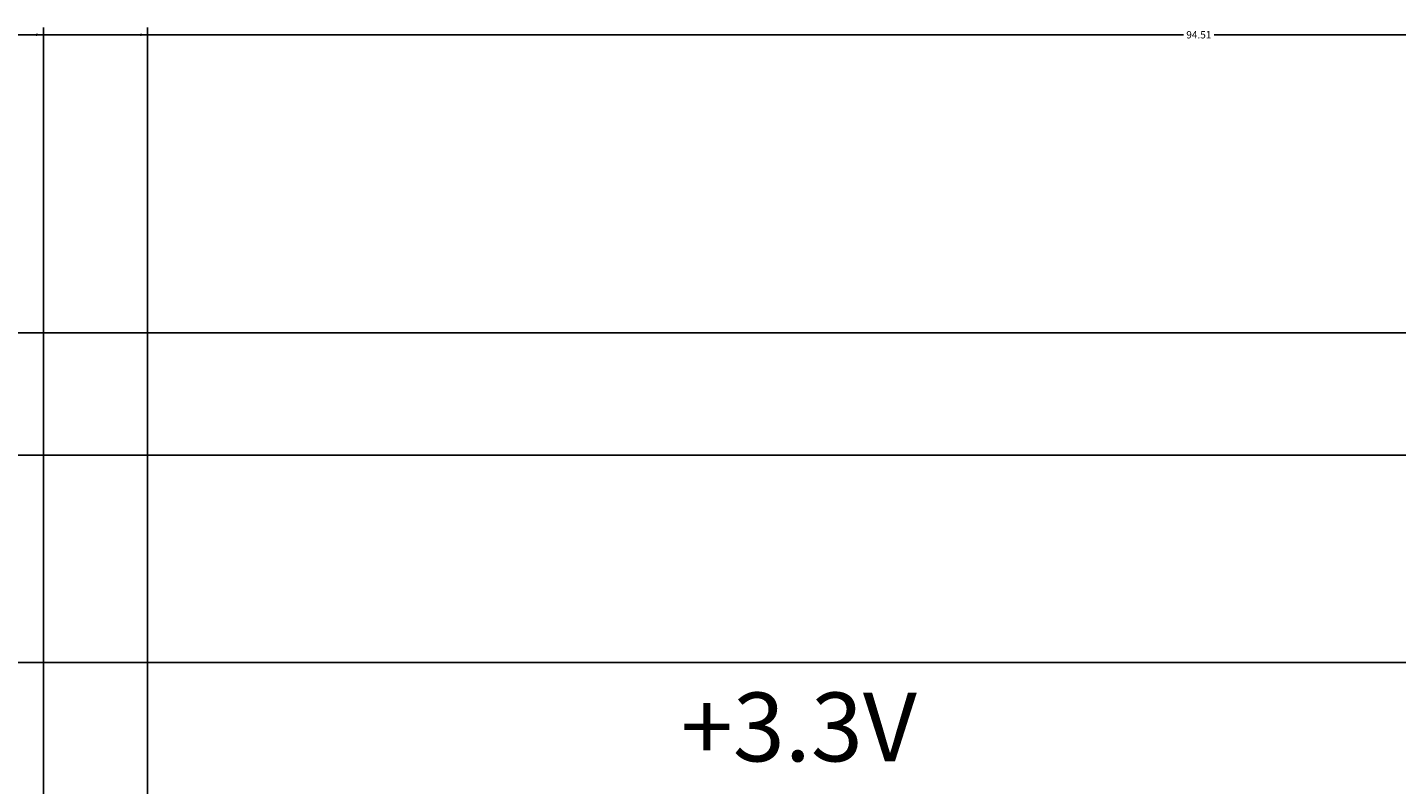
# Model space of a CAD drawing. Units: inches. Extents: x 23 to 132, y 5 to 105.
# Tile 6 of 14: x 47 to 81, y 87 to 105. Entities that reach past the tile are written whole.
import ezdxf

# ---------------------------------------------------------------- set-up
doc = ezdxf.new("R2010")
doc.units = ezdxf.units.IN
doc.header["$MEASUREMENT"] = 0
doc.layers.add('A-ANNO-DIMS', color=2, linetype='Continuous', lineweight=18)
doc.layers.add('E-ANNO-IDEN', color=4, linetype='Continuous', lineweight=18)
doc.styles.get("Standard").update_dxf_attribs({"font": 'arial.ttf'})
doc.dimstyles.get("Standard").update_dxf_attribs({"dimtxt": 0.18, "dimasz": 0.18, "dimexe": 0.18, "dimexo": 0.0625, "dimgap": 0.09, "dimtad": 0, "dimtih": 1, "dimtoh": 1, "dimdec": 4, "dimzin": 0, "dimdsep": 46, "dimtxsty": 'Standard', "dimcen": 0.09, "dimadec": 0, "dimazin": 0, "dimtfac": 1, "dimtdec": 4, "dimtofl": 0, "dimtmove": 0, "dimatfit": 3, "dimfxl": 1, "dimtolj": 1, "dimtzin": 0, "dimarcsym": 0})

# ---------------------------------------------------------------- blocks, each defined once
blk = doc.blocks.new('*D2')
at = {"layer": 'A-ANNO-DIMS', "color": 0, "lineweight": -2, "transparency": 16777216}
for p, q in [((28.697, 66.272), (28.697, 105.232)), ((123.211, 99.539), (123.211, 105.232)), ((28.877, 105.052), (75.577, 105.052)), ((123.031, 105.052), (76.33, 105.052))]:
    blk.add_line(p, q, dxfattribs=at)
at = {"layer": 'A-ANNO-DIMS', "color": 0, "transparency": 16777216}
for points in [[(28.877, 105.082), (28.877, 105.022), (28.697, 105.052)], [(123.031, 105.082), (123.031, 105.022), (123.211, 105.052)]]:
    blk.add_solid(points, dxfattribs=at)
at = {"layer": 'Defpoints', "color": 0, "transparency": 16777216}
for p in [(123.211, 105.052), (123.211, 99.477), (28.697, 66.21)]:
    blk.add_point(p, dxfattribs=at)
at = {"layer": 'A-ANNO-DIMS', "color": 0, "transparency": 16777216, "insert": (75.954, 105.052), "char_height": 0.18, "attachment_point": 5}
blk.add_mtext('\\A1;94.51', dxfattribs=at)
blk = doc.blocks.new('*D3')
at = {"layer": 'A-ANNO-DIMS', "color": 0, "lineweight": -2, "transparency": 16777216}
for p, q in [((121.409, 99.285), (129.239, 99.285)), ((129.059, 99.105), (129.059, 55.423)), ((129.059, 11.378), (129.059, 55.06)), ((72.981, 11.198), (129.239, 11.198))]:
    blk.add_line(p, q, dxfattribs=at)
at = {"layer": 'A-ANNO-DIMS', "color": 0, "transparency": 16777216}
for points in [[(129.029, 99.105), (129.089, 99.105), (129.059, 99.285)], [(129.029, 11.378), (129.089, 11.378), (129.059, 11.198)]]:
    blk.add_solid(points, dxfattribs=at)
at = {"layer": 'Defpoints', "color": 0, "transparency": 16777216}
for p in [(121.346, 99.285), (129.059, 99.285), (72.919, 11.198)]:
    blk.add_point(p, dxfattribs=at)
at = {"layer": 'A-ANNO-DIMS', "color": 0, "transparency": 16777216, "insert": (129.059, 55.241), "char_height": 0.18, "attachment_point": 5}
blk.add_mtext('\\A1;88.09', dxfattribs=at)
blk = doc.blocks.new('*D7')
at = {"layer": 'A-ANNO-DIMS', "color": 0, "lineweight": -2, "transparency": 16777216}
for p, q in [((30.295, 73.877), (30.295, 105.232)), ((50.265, 77.157), (50.265, 105.232)), ((30.475, 105.052), (39.895, 105.052)), ((50.085, 105.052), (40.665, 105.052))]:
    blk.add_line(p, q, dxfattribs=at)
at = {"layer": 'A-ANNO-DIMS', "color": 0, "transparency": 16777216}
for points in [[(30.475, 105.082), (30.475, 105.022), (30.295, 105.052)], [(50.085, 105.082), (50.085, 105.022), (50.265, 105.052)]]:
    blk.add_solid(points, dxfattribs=at)
at = {"layer": 'Defpoints', "color": 0, "transparency": 16777216}
for p in [(50.265, 105.052), (50.265, 77.095), (30.295, 73.814)]:
    blk.add_point(p, dxfattribs=at)
at = {"layer": 'A-ANNO-DIMS', "color": 0, "transparency": 16777216, "insert": (40.28, 105.052), "char_height": 0.18, "attachment_point": 5}
blk.add_mtext('\\A1;19.97', dxfattribs=at)
blk = doc.blocks.new('*D48')
at = {"layer": 'A-ANNO-DIMS', "color": 0, "lineweight": -2, "transparency": 16777216}
for p, q in [((41.783, 75.637), (41.783, 105.232)), ((47.72, 75.683), (47.72, 105.232)), ((41.963, 105.052), (44.358, 105.052)), ((47.54, 105.052), (45.145, 105.052))]:
    blk.add_line(p, q, dxfattribs=at)
at = {"layer": 'A-ANNO-DIMS', "color": 0, "transparency": 16777216}
for points in [[(41.963, 105.082), (41.963, 105.022), (41.783, 105.052)], [(47.54, 105.082), (47.54, 105.022), (47.72, 105.052)]]:
    blk.add_solid(points, dxfattribs=at)
at = {"layer": 'Defpoints', "color": 0, "transparency": 16777216}
for p in [(47.72, 105.052), (41.783, 75.575), (47.72, 75.621)]:
    blk.add_point(p, dxfattribs=at)
at = {"layer": 'A-ANNO-DIMS', "color": 0, "transparency": 16777216, "insert": (44.752, 105.052), "char_height": 0.18, "attachment_point": 5}
blk.add_mtext('\\A1;5.937', dxfattribs=at)
blk = doc.blocks.new('*D85')
at = {"layer": 'A-ANNO-DIMS', "color": 0, "lineweight": -2, "transparency": 16777216}
for p, q in [((106.903, 97.776), (22.942, 97.776)), ((23.122, 97.596), (23.122, 87.606)), ((23.122, 77.251), (23.122, 87.242)), ((106.964, 77.071), (22.942, 77.071))]:
    blk.add_line(p, q, dxfattribs=at)
at = {"layer": 'A-ANNO-DIMS', "color": 0, "transparency": 16777216}
for points in [[(23.092, 97.596), (23.152, 97.596), (23.122, 97.776)], [(23.092, 77.251), (23.152, 77.251), (23.122, 77.071)]]:
    blk.add_solid(points, dxfattribs=at)
at = {"layer": 'Defpoints', "color": 0, "transparency": 16777216}
for p in [(23.122, 97.776), (106.965, 97.776), (107.026, 77.071)]:
    blk.add_point(p, dxfattribs=at)
at = {"layer": 'A-ANNO-DIMS', "color": 0, "transparency": 16777216, "insert": (23.122, 87.424), "char_height": 0.18, "attachment_point": 5}
blk.add_mtext('\\A1;20.705', dxfattribs=at)
blk = doc.blocks.new('*D88')
at = {"layer": 'A-ANNO-DIMS', "color": 0, "lineweight": -2, "transparency": 16777216}
for p, q in [((110.027, 89.722), (22.942, 89.722)), ((23.122, 89.542), (23.122, 87.554)), ((23.122, 85.201), (23.122, 87.19)), ((110.027, 85.021), (22.942, 85.021))]:
    blk.add_line(p, q, dxfattribs=at)
at = {"layer": 'A-ANNO-DIMS', "color": 0, "transparency": 16777216}
for points in [[(23.092, 89.542), (23.152, 89.542), (23.122, 89.722)], [(23.092, 85.201), (23.152, 85.201), (23.122, 85.021)]]:
    blk.add_solid(points, dxfattribs=at)
at = {"layer": 'Defpoints', "color": 0, "transparency": 16777216}
for p in [(23.122, 89.722), (110.089, 89.722), (110.089, 85.021)]:
    blk.add_point(p, dxfattribs=at)
at = {"layer": 'A-ANNO-DIMS', "color": 0, "transparency": 16777216, "insert": (23.122, 87.372), "char_height": 0.18, "attachment_point": 5}
blk.add_mtext('\\A1;4.702', dxfattribs=at)
blk = doc.blocks.new('*D89')
at = {"layer": 'A-ANNO-DIMS', "color": 0, "lineweight": -2, "transparency": 16777216}
for p, q in [((110.298, 94.783), (22.942, 94.783)), ((23.122, 94.603), (23.122, 92.435)), ((23.122, 89.902), (23.122, 92.071)), ((110.027, 89.722), (22.942, 89.722))]:
    blk.add_line(p, q, dxfattribs=at)
at = {"layer": 'A-ANNO-DIMS', "color": 0, "transparency": 16777216}
for points in [[(23.092, 94.603), (23.152, 94.603), (23.122, 94.783)], [(23.092, 89.902), (23.152, 89.902), (23.122, 89.722)]]:
    blk.add_solid(points, dxfattribs=at)
at = {"layer": 'Defpoints', "color": 0, "transparency": 16777216}
for p in [(23.122, 94.783), (110.36, 94.783), (110.089, 89.722)]:
    blk.add_point(p, dxfattribs=at)
at = {"layer": 'A-ANNO-DIMS', "color": 0, "transparency": 16777216, "insert": (23.122, 92.253), "char_height": 0.18, "attachment_point": 5}
blk.add_mtext('\\A1;5.061', dxfattribs=at)
blk = doc.blocks.new('*D90')
at = {"layer": 'A-ANNO-DIMS', "color": 0, "lineweight": -2, "transparency": 16777216}
for p, q in [((106.903, 97.776), (22.942, 97.776)), ((23.122, 97.596), (23.122, 96.462)), ((23.122, 94.963), (23.122, 96.098)), ((110.298, 94.783), (22.942, 94.783))]:
    blk.add_line(p, q, dxfattribs=at)
at = {"layer": 'A-ANNO-DIMS', "color": 0, "transparency": 16777216}
for points in [[(23.092, 97.596), (23.152, 97.596), (23.122, 97.776)], [(23.092, 94.963), (23.152, 94.963), (23.122, 94.783)]]:
    blk.add_solid(points, dxfattribs=at)
at = {"layer": 'Defpoints', "color": 0, "transparency": 16777216}
for p in [(23.122, 97.776), (106.965, 97.776), (110.36, 94.783)]:
    blk.add_point(p, dxfattribs=at)
at = {"layer": 'A-ANNO-DIMS', "color": 0, "transparency": 16777216, "insert": (23.122, 96.28), "char_height": 0.18, "attachment_point": 5}
blk.add_mtext('\\A1;2.993', dxfattribs=at)

msp = doc.modelspace()

# ---------------------------------------------------------------- texts
at = {"layer": 'E-ANNO-IDEN'}
msp.add_text('+3.3V', height=1.67943, dxfattribs=at).set_placement((63.2927, 87.3072))

# ---------------------------------------------------------------- dimensions: what is measured, and where the dimension line sits
at = {"layer": 'A-ANNO-DIMS'}
for base, p1, p2, override, picture, middle in [((123.2107, 105.052), (28.6965, 66.2099), (123.2107, 99.477), {"dimdec": 2, "dimlfac": 1, "dimrnd": 0, "dimzin": 0, "dimdsep": 46, "dimlunit": 2}, '*D2', (75.9536, 105.052)), ((50.2646, 105.052), (30.2954, 73.8144), (50.2646, 77.095), {"dimdec": 2, "dimlfac": 1, "dimrnd": 0, "dimzin": 0, "dimdsep": 46, "dimlunit": 2}, '*D7', (40.28, 105.052)), ((47.7202, 105.052), (41.7829, 75.5745), (47.7202, 75.6207), {"dimdec": 3, "dimlfac": 1, "dimrnd": 0, "dimzin": 0, "dimdsep": 46, "dimlunit": 2}, '*D48', (44.7515, 105.052))]:
    dim = msp.add_linear_dim(base=base, p1=p1, p2=p2, dimstyle='Standard', override=override, dxfattribs=at)
    dim.commit()
    dim.dimension.update_dxf_attribs({"geometry": picture, "text_midpoint": middle})
for base, p1, p2, override, picture, middle in [((129.0589, 99.2846), (72.9188, 11.1983), (121.3461, 99.2846), {"dimdec": 2, "dimlfac": 1, "dimrnd": 0, "dimzin": 0, "dimdsep": 46, "dimlunit": 2}, '*D3', (129.0589, 55.2415)), ((23.1215, 97.7764), (107.026, 77.0711), (106.9652, 97.7764), {"dimdec": 3, "dimlfac": 1, "dimrnd": 0, "dimzin": 0, "dimdsep": 46, "dimlunit": 2}, '*D85', (23.1215, 87.4238)), ((23.1215, 97.7764), (110.36, 94.7833), (106.9652, 97.7764), {"dimdec": 3, "dimlfac": 1, "dimrnd": 0, "dimzin": 0, "dimdsep": 46, "dimlunit": 2}, '*D90', (23.1215, 96.2798)), ((23.1215, 94.7833), (110.0892, 89.7224), (110.36, 94.7833), {"dimdec": 3, "dimlfac": 1, "dimrnd": 0, "dimzin": 0, "dimdsep": 46, "dimlunit": 2}, '*D89', (23.1215, 92.2528)), ((23.12152, 89.7224), (110.08916, 85.02085), (110.08916, 89.7224), {"dimdec": 3, "dimlfac": 1, "dimrnd": 0, "dimzin": 0, "dimdsep": 46, "dimlunit": 2}, '*D88', (23.12152, 87.37162))]:
    dim = msp.add_linear_dim(base=base, p1=p1, p2=p2, angle=90, dimstyle='Standard', override=override, dxfattribs=at)
    dim.commit()
    dim.dimension.update_dxf_attribs({"geometry": picture, "text_midpoint": middle})

doc.saveas('drawing.dxf')
